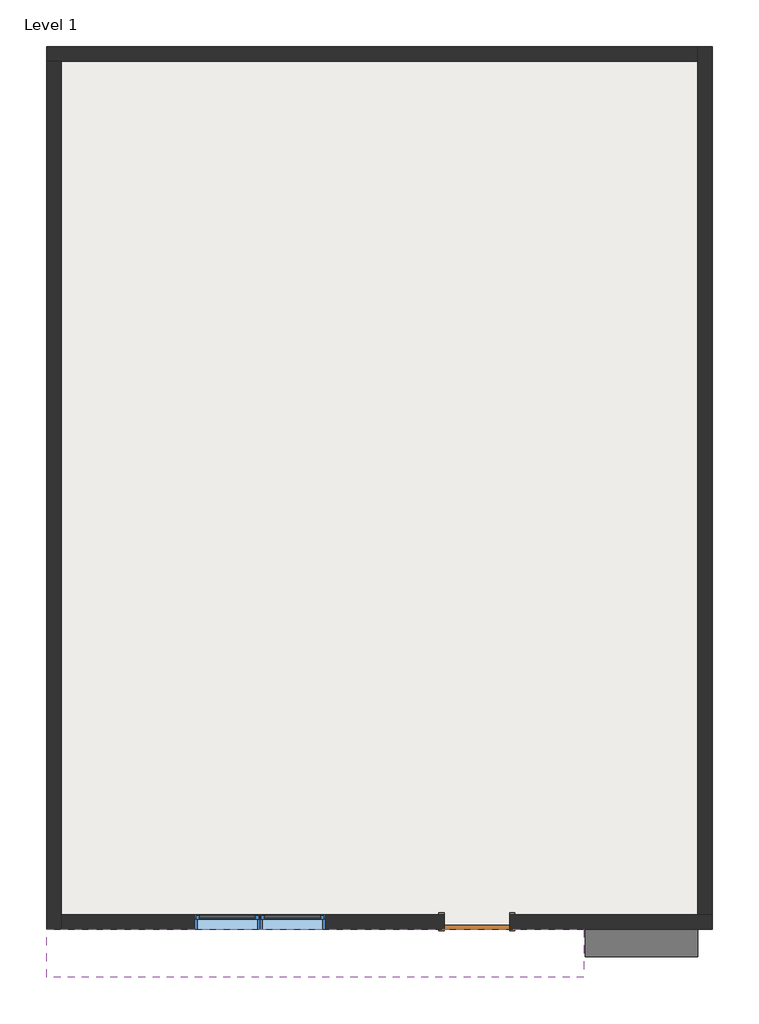
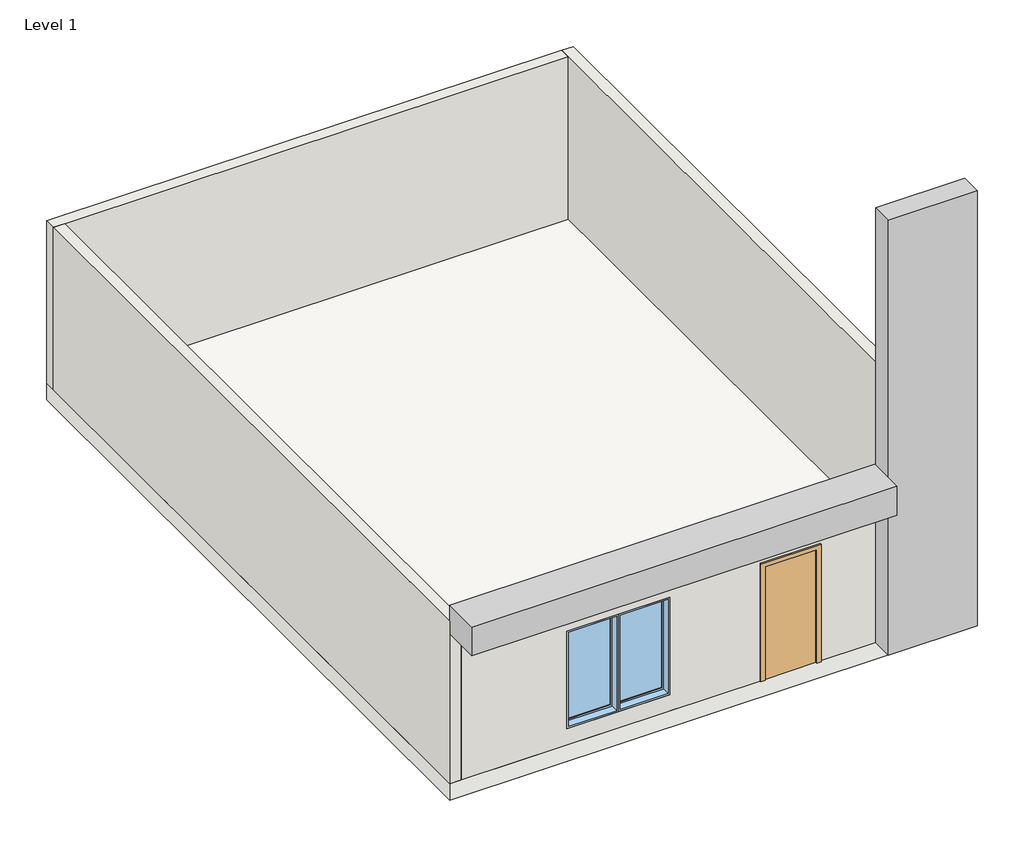
# One storey: 4 walls, 2 proxies, 2 windows, 1 door, 1 slab.
"""IFC4 building model written with IfcOpenShell, lengths in millimetres."""

from ifc_helpers import new_model, si_unit, frame, origin, place, context, project, spatial, polyline, outline, extrude, faceted_brep, transform, mapped, element, save
from components import generic_models_1_generic_models_1_d491554d, generic_models_2_generic_models_2_34e4dd5e, door_719f80de, window_9a779fa2

model = new_model("IFC4")

# Units and contexts
model_context = context("Model", 3, world=origin())
ifc_project = project(units=[si_unit("LENGTHUNIT", "METRE", prefix="MILLI")], contexts=[model_context])

# Site, building, storey
site = spatial("IfcSite", under=ifc_project)
building = spatial("IfcBuilding", under=site)
storey = spatial("IfcBuildingStorey", under=building, Name="Level 1", Elevation=0.0)

# Proxies
placement = place(None, origin())
generic_models_1_generic_models_1_shape = generic_models_1_generic_models_1_d491554d(model_context)
element("IfcBuildingElementProxy", 1, Name="Generic Models 1 : Generic Models 1", ObjectType="Generic Models 1 : Generic Models 1", at=placement, inside=storey, context=model_context, shape_type="MappedRepresentation", body=[
    mapped(generic_models_1_generic_models_1_shape, transform((0.0, 0.0, 0.0), x_axis=(1.0, 0.0, 0.0), y_axis=(0.0, 1.0, 0.0), z_axis=(0.0, 0.0, 1.0))),
])
generic_models_2_generic_models_2_shape = generic_models_2_generic_models_2_34e4dd5e(model_context)
element("IfcBuildingElementProxy", 2, Name="Generic Models 2 : Generic Models 2", ObjectType="Generic Models 2 : Generic Models 2", at=placement, inside=storey, context=model_context, shape_type="MappedRepresentation", body=[
    mapped(generic_models_2_generic_models_2_shape, transform((0.0, 0.0, 0.0), x_axis=(1.0, 0.0, 0.0), y_axis=(0.0, 1.0, 0.0), z_axis=(0.0, 0.0, 1.0))),
])

# Door
door_shape = door_719f80de(model_context)
element("IfcDoor", 3, ObjectType="Single-Flush : 36\" x 84\"", at=placement, inside=storey, context=model_context, shape_type="MappedRepresentation", body=[
    mapped(door_shape, transform((-4461.6128458, 1953.219734, 0.0), x_axis=(1.0, 0.0, 0.0), y_axis=(0.0, 1.0, 0.0), z_axis=(0.0, 0.0, 1.0))),
])

# Slab
element("IfcSlab", 4, ObjectType="Generic - 12\"", at=placement, inside=storey, context=model_context, shape_type="SweptSolid", body=[
    extrude(outline(polyline([(-1159.6128458, 14246.819734), (-1159.6128458, 1851.619734), (-10506.8128458, 1851.619734), (-10506.8128458, 14246.819734), (-1159.6128458, 14246.819734)])), frame((0.0, 0.0, -304.8), z_axis=(0.0, 0.0, 1.0), x_axis=(1.0, 0.0, 0.0)), (0.0, 0.0, 1.0), 304.8),
])

# Walls
element("IfcWall", 5, ObjectType="Generic - 8\"", at=placement, inside=storey, context=model_context, shape_type="Brep", body=[
    faceted_brep([(-10506.8128458, 14043.619734, 0.0), (-10303.6128458, 14043.619734, 0.0), (-1362.8128458, 14043.619734, 0.0), (-1362.8128458, 14043.619734, 3048.0), (-10303.6128458, 14043.619734, 3048.0), (-10506.8128458, 14043.619734, 3048.0), (-10506.8128458, 14246.819734, 0.0), (-10506.8128458, 14246.819734, 3048.0), (-1362.8128458, 14246.819734, 3048.0), (-1362.8128458, 14246.819734, 0.0)], [[[0, 1, 2, 3, 4, 5]], [[6, 7, 8, 9]], [[2, 1, 0, 6, 9]], [[0, 5, 7, 6]], [[3, 2, 9, 8]], [[5, 4, 3, 8, 7]]]),
])
element("IfcWall", 6, ObjectType="Generic - 8\"", at=placement, inside=storey, context=model_context, shape_type="Brep", body=[
    faceted_brep([(-10303.6128458, 1851.619734, 0.0), (-10303.6128458, 2054.819734, 0.0), (-10303.6128458, 14043.619734, 0.0), (-10303.6128458, 14043.619734, 3048.0), (-10303.6128458, 2054.819734, 3048.0), (-10303.6128458, 1851.619734, 3048.0), (-10506.8128458, 1851.619734, 0.0), (-10506.8128458, 1851.619734, 3048.0), (-10506.8128458, 14043.619734, 3048.0), (-10506.8128458, 14043.619734, 0.0)], [[[0, 1, 2, 3, 4, 5]], [[6, 7, 8, 9]], [[2, 1, 0, 6, 9]], [[0, 5, 7, 6]], [[3, 2, 9, 8]], [[5, 4, 3, 8, 7]]]),
])
element("IfcWall", 7, ObjectType="Generic - 8\"", at=placement, inside=storey, context=model_context, shape_type="Brep", body=[
    faceted_brep([(-1159.6128458, 2054.819734, 3048.0), (-1159.6128458, 2054.819734, 0.0), (-1362.8128458, 2054.819734, 0.0), (-4004.4128458, 2054.819734, 0.0), (-4004.4128458, 2054.819734, 2133.6), (-4918.8128458, 2054.819734, 2133.6), (-4918.8128458, 2054.819734, 0.0), (-10303.6128458, 2054.819734, 0.0), (-10303.6128458, 2054.819734, 3048.0), (-1362.8128458, 2054.819734, 3048.0), (-8424.0128458, 2054.819734, 304.8), (-6595.2128458, 2054.819734, 304.8), (-6595.2128458, 2054.819734, 2133.6), (-8424.0128458, 2054.819734, 2133.6), (-1159.6128458, 1851.619734, 0.0), (-1159.6128458, 1851.619734, 3048.0), (-10303.6128458, 1851.619734, 3048.0), (-10303.6128458, 1851.619734, 0.0), (-4918.8128458, 1851.619734, 0.0), (-4918.8128458, 1851.619734, 2133.6), (-4004.4128458, 1851.619734, 2133.6), (-4004.4128458, 1851.619734, 0.0), (-6595.2128458, 1851.619734, 304.8), (-8424.0128458, 1851.619734, 304.8), (-8424.0128458, 1851.619734, 2133.6), (-6595.2128458, 1851.619734, 2133.6)], [[[0, 1, 2, 3, 4, 5, 6, 7, 8, 9], [10, 11, 12, 13]], [[14, 15, 16, 17, 18, 19, 20, 21], [22, 23, 24, 25]], [[1, 14, 21, 3, 2]], [[17, 7, 6, 18]], [[1, 0, 15, 14]], [[8, 7, 17, 16]], [[0, 9, 8, 16, 15]], [[4, 3, 21, 20]], [[5, 4, 20, 19]], [[6, 5, 19, 18]], [[22, 11, 10, 23]], [[24, 23, 10, 13]], [[24, 13, 12, 25]], [[25, 12, 11, 22]]]),
])
element("IfcWall", 8, ObjectType="Generic - 8\"", at=placement, inside=storey, context=model_context, shape_type="Brep", body=[
    faceted_brep([(-1362.8128458, 14246.819734, 0.0), (-1362.8128458, 14043.619734, 0.0), (-1362.8128458, 2054.819734, 0.0), (-1362.8128458, 2054.819734, 3048.0), (-1362.8128458, 14043.619734, 3048.0), (-1362.8128458, 14246.819734, 3048.0), (-1159.6128458, 14246.819734, 0.0), (-1159.6128458, 14246.819734, 3048.0), (-1159.6128458, 2054.819734, 3048.0), (-1159.6128458, 2054.819734, 0.0)], [[[0, 1, 2, 3, 4, 5]], [[6, 7, 8, 9]], [[2, 1, 0, 6, 9]], [[0, 5, 7, 6]], [[3, 2, 9, 8]], [[5, 4, 3, 8, 7]]]),
])

# Windows
window_shape = window_9a779fa2(model_context)
element("IfcWindow", 9, ObjectType="Fixed : 36\" x 72\"", at=placement, inside=storey, context=model_context, shape_type="MappedRepresentation", body=[
    mapped(window_shape, transform((-7928.7128458, 1953.219734, 0.0), x_axis=(1.0, 0.0, 0.0), y_axis=(0.0, 1.0, 0.0), z_axis=(0.0, 0.0, 1.0))),
])
element("IfcWindow", 10, ObjectType="Fixed : 36\" x 72\"", at=placement, inside=storey, context=model_context, shape_type="MappedRepresentation", body=[
    mapped(window_shape, transform((-7014.3128458, 1953.219734, 0.0), x_axis=(1.0, 0.0, 0.0), y_axis=(0.0, 1.0, 0.0), z_axis=(0.0, 0.0, 1.0))),
])

save(model, "model.ifc")

# Revit data of these elements
# Type "Single-Flush : 36\" x 84\""
#   Type Mark = "1"
#   Construction Type Id = "MDOOR"
#   Assembly Code = "C1020"
#   Analytic Construction = "Metal"
#   Thickness = 0' - 2"
#   Heat Transfer Coefficient (U) = 0.651978 BTU/(h·ft²·°F)
#   Height = 7' - 0"
#   Trim Projection Ext = 0' - 1"
#   Trim Projection Int = 0' - 1"
#   Trim Width = 0' - 3"
#   Width = 3' - 0"
#   Define Thermal Properties by = 1
#   Door Material = Door - Panel
#   Frame Material = Door - Frame
#   Visual Light Transmittance = 0
#   Solar Heat Gain Coefficient = 0
#   Function = (empty or 0)
#   Wall Closure = (empty or 0)
# Type "Generic - 12\""
#   Assembly Code = "B1010"
#   Function = 0
#   Layers, outside or top first: 1' - 0" no material (function 1)
# Type "Generic - 8\""
#   Assembly Code = "B2010"
#   Layers, outside or top first: 0' - 8" no material (function 1)
# Type "Fixed : 36\" x 72\""
#   Type Mark = "9"
#   Construction Type Id = "GSP4R"
#   Assembly Code = "B2020100"
#   Analytic Construction = "1/8 in Pilkington single glazing"
#   Visual Light Transmittance = 0.9
#   Solar Heat Gain Coefficient = 0.78
#   Heat Transfer Coefficient (U) = 0.6496 BTU/(h·ft²·°F)
#   Height = 6' - 0"
#   Default Sill Height = 1' - 0"
#   Width = 3' - 0"
#   Window Inset = 0' - 0 3/4"
#   Define Thermal Properties by = 1
#   Glass Pane Material = Glass
#   Sash Material = Sash
#   Wall Closure = (empty or 0)
# Element 1 (IfcBuildingElementProxy, "Generic Models 1 : Generic Models 1")
#   Phase Created = New Construction
# Element 2 (IfcBuildingElementProxy, "Generic Models 2 : Generic Models 2")
#   Phase Created = New Construction
# Element 3 (IfcDoor, "Single-Flush : 36\" x 84\"")
#   Phase Created = New Construction
#   Materials on its faces: "Door - Frame", "Door - Panel"
# Element 4 (IfcSlab, "Generic - 12\"")
#   Height Offset From Level = 0' - 0"
#   Phase Created = New Construction
#   Materials on its faces: "Default Floor"
# Elements 5, 6, 7, 8 (IfcWall, "Generic - 8\"")
#   Top Offset = 0' - 0"
#   Base Offset = 0' - 0"
#   Unconnected Height = 10' - 0"
#   wall height = 10' - 0"
#   Phase Created = New Construction
#   Base Constraint = Level 1
#   Materials on its faces: "Default Wall"
# Element 9 (IfcWindow, "Fixed : 36\" x 72\"")
#   Mark = "1"
#   Phase Created = New Construction
#   Materials on its faces: "Sash", "Glass"
# Element 10 (IfcWindow, "Fixed : 36\" x 72\"")
#   Mark = "4"
#   Phase Created = New Construction
#   Materials on its faces: "Sash", "Glass"
# Materials
#   "Door - Panel": class "Wood", colour RGB 210 159 95, transparency 0
#   "Door - Frame": colour RGB 118 70 51, transparency 0
#   "Glass": class "Glass", colour RGB 0 128 192, transparency 0.75, Description = "Soda Lime Glass", Cost = 0
#   "Sash": class "Wood", colour RGB 224 178 126, transparency 0
#   "Default Floor": colour RGB 128 128 128, transparency 0
#   "Default Wall": colour RGB 128 128 128, transparency 0
